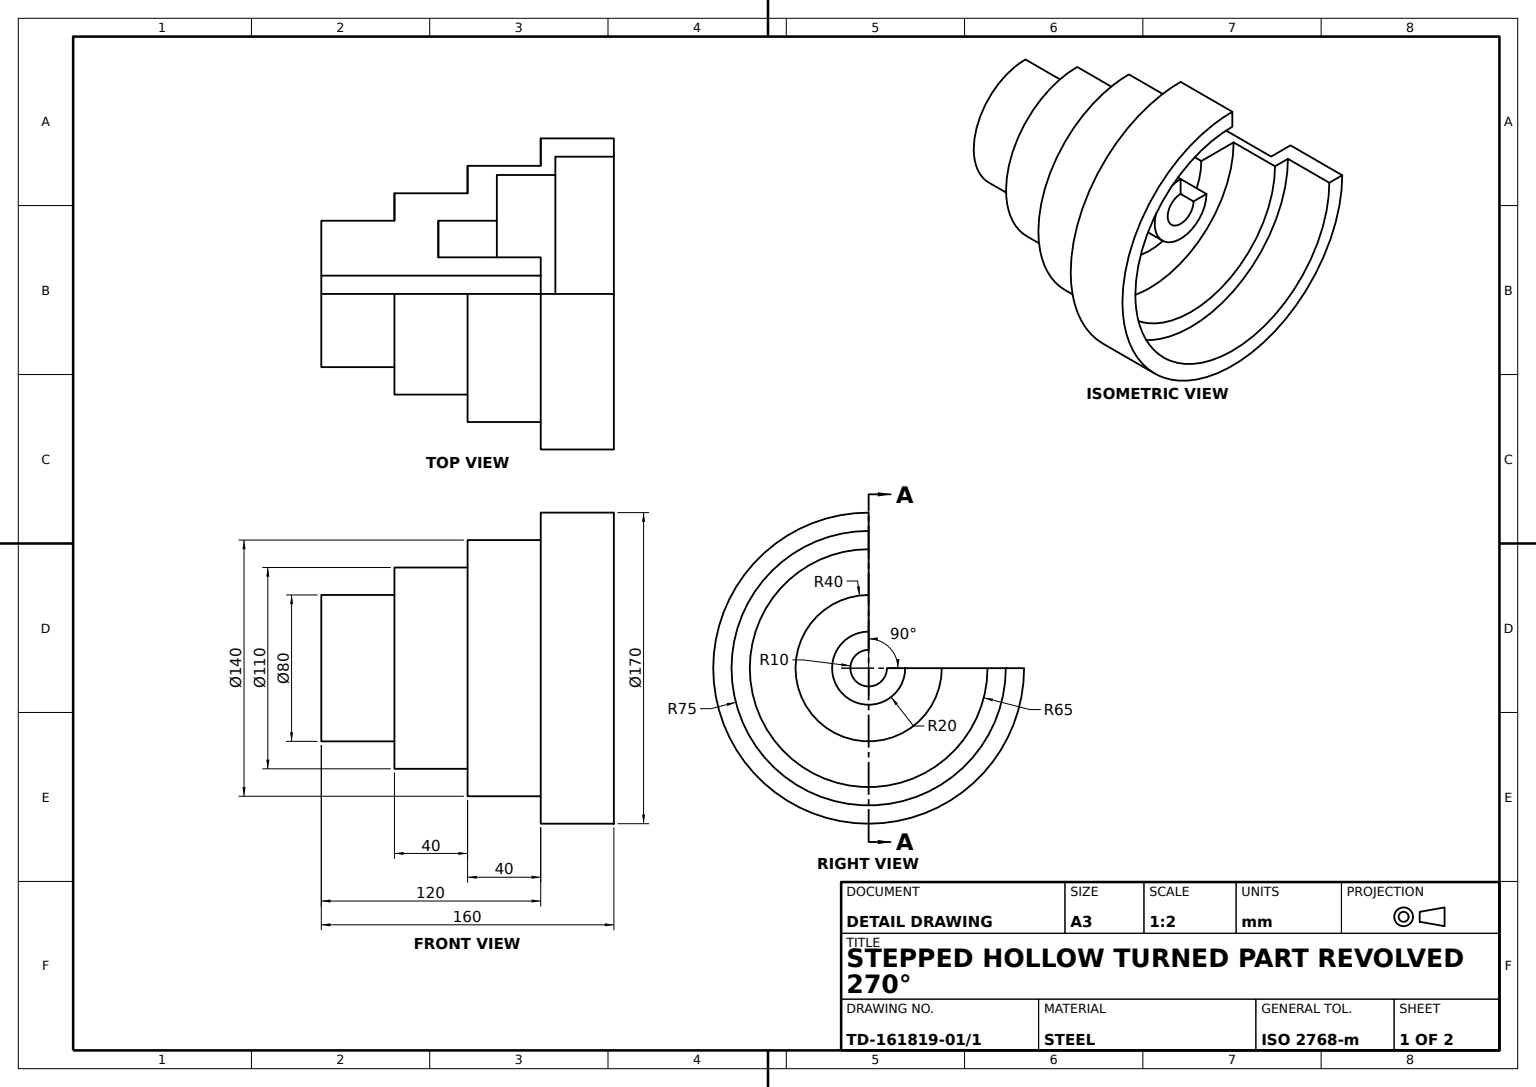
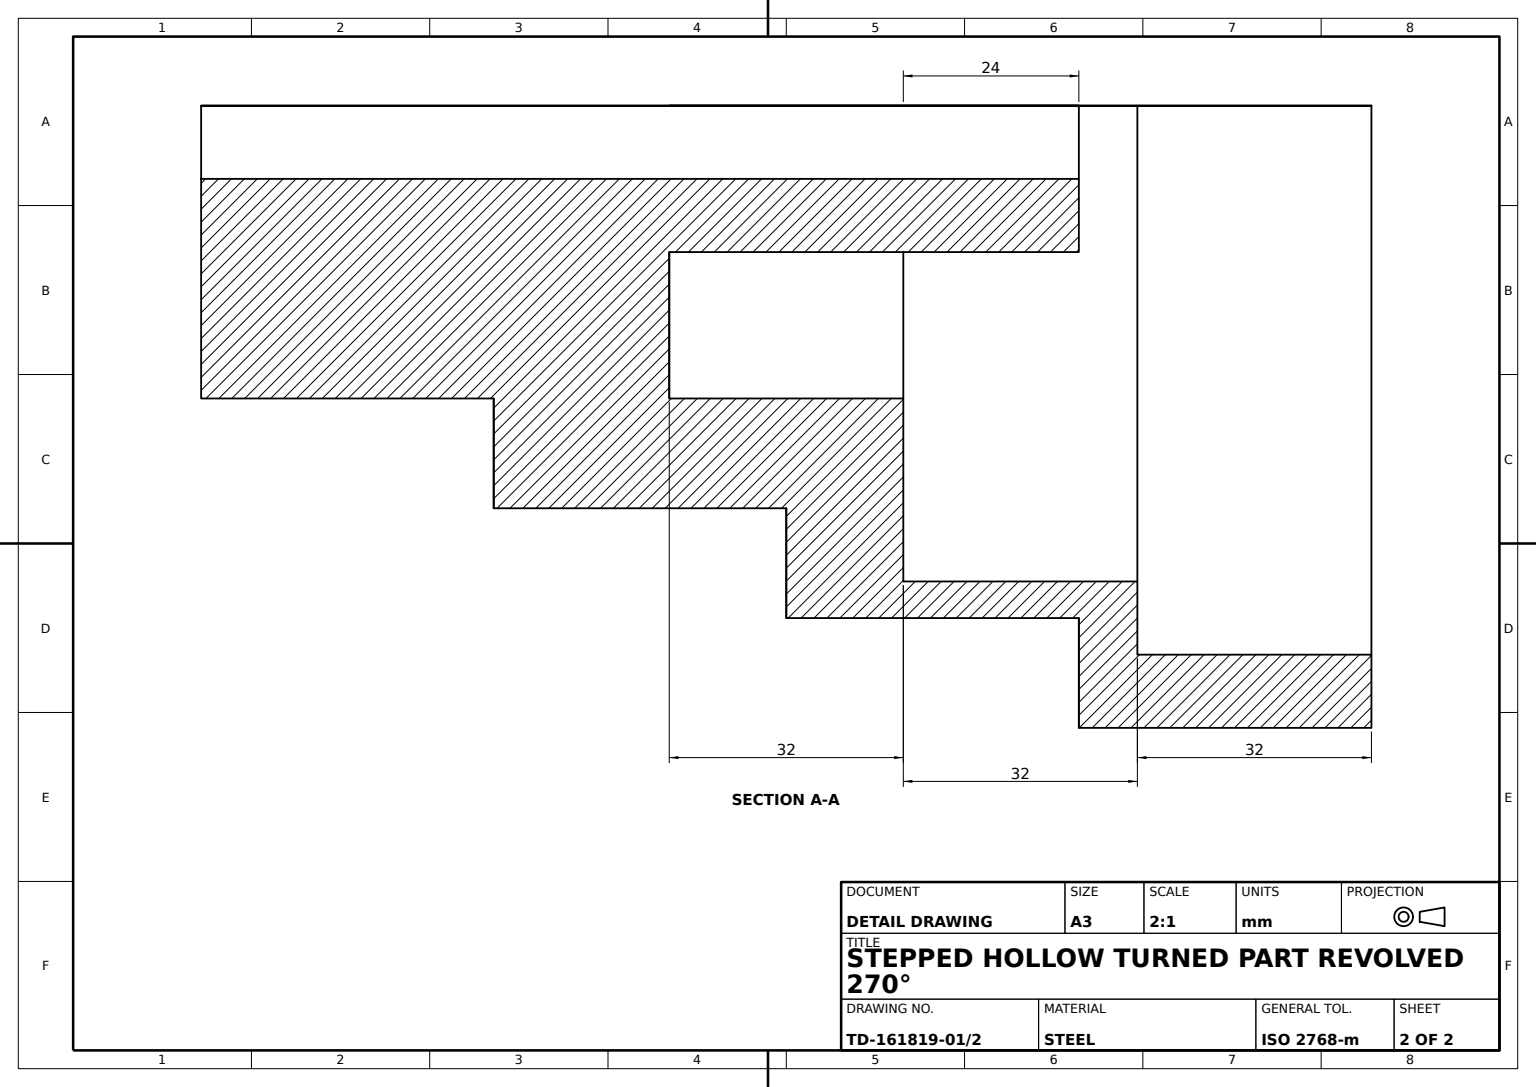
SolidWorks part; units mm, degrees
material "Plain Carbon Steel"
ref_plane "Front Plane" through (0, 0, 0) normal (0, 0, 1) x (1, 0, 0)
ref_plane "Top Plane" through (0, 0, 0) normal (0, 1, 0) x (1, 0, 0)
ref_plane "Right Plane" through (0, 0, 0) normal (1, 0, 0) x (0, 0, -1)
sketch "Stepped Housing Profile" plane through (0, 0, 0) normal (0, 0, 1) x (1, 0, 0)
  line L0 (0, 0) -> (0, 40)
  line L1 (0, 40) -> (40, 40)
  line L2 (40, 40) -> (40, 55)
  line L3 (40, 55) -> (80, 55)
  line L4 (80, 55) -> (80, 70)
  line L5 (80, 70) -> (120, 70)
  line L6 (120, 70) -> (120, 85)
  line L7 (120, 85) -> (160, 85)
  line L10 (0, 0) -> (160, 0) construction
  line L11 (160, 85) -> (160, 75)
  line L21 (0, 0) -> (120, 0)
  line L22 (160, 75) -> (128, 75)
  line L23 (128, 75) -> (128, 65)
  line L24 (128, 65) -> (96, 65)
  line L25 (96, 65) -> (96, 40)
  line L26 (96, 40) -> (64, 40)
  line L27 (64, 40) -> (64, 20)
  line L28 (64, 20) -> (120, 20)
  line L29 (120, 20) -> (120, 10)
  line L30 (120, 10) -> (0, 10)
  line L31 (0, 10) -> (0, 40)
  dimension "D1" = 40
  dimension "D2" = 40
  dimension "D3" = 10
  dimension "D4" = 55
  dimension "D5" = 70
  dimension "D6" = 85
  dimension "D7" = 32
  dimension "D8" = 32
  dimension "D9" = 32
  dimension "D10" = 30
  dimension "D11" = 10
  dimension "D12" = 10
  dimension "D13" = 120
revolve "Housing Revolve 270deg" add sketch "Stepped Housing Profile" angle 270 about L10
